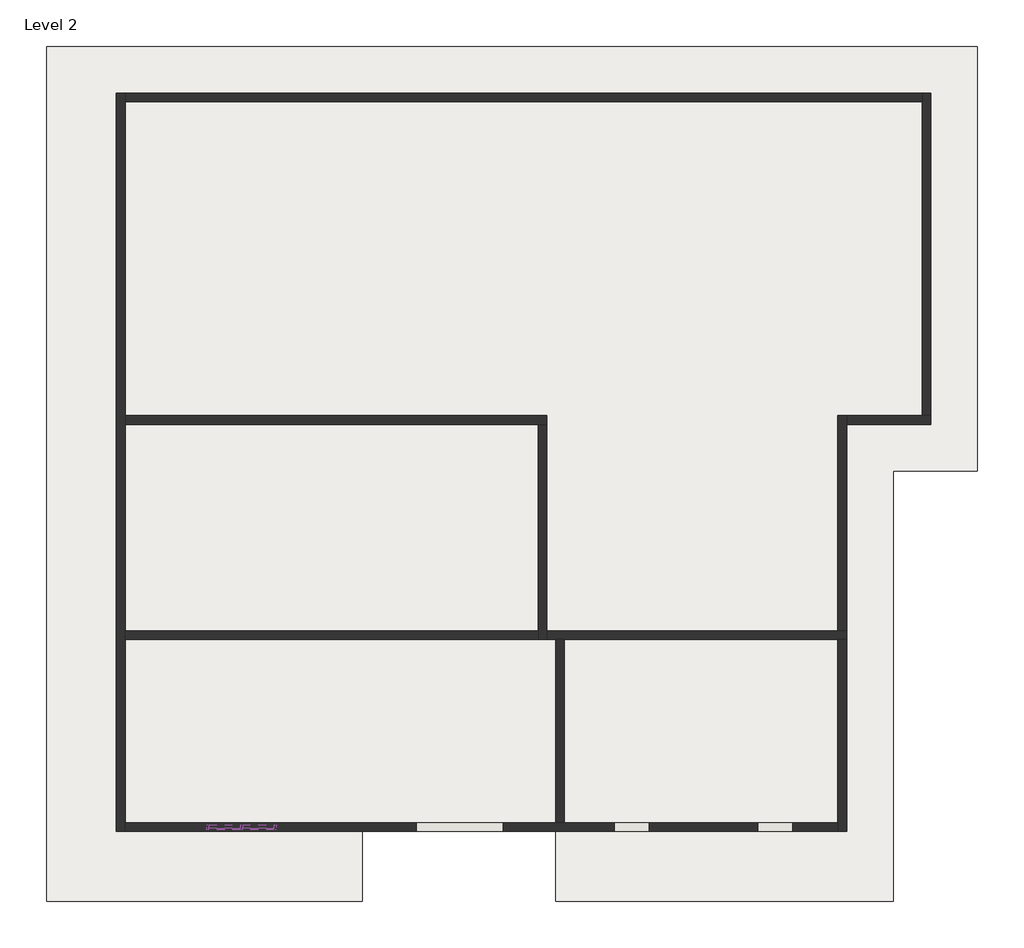
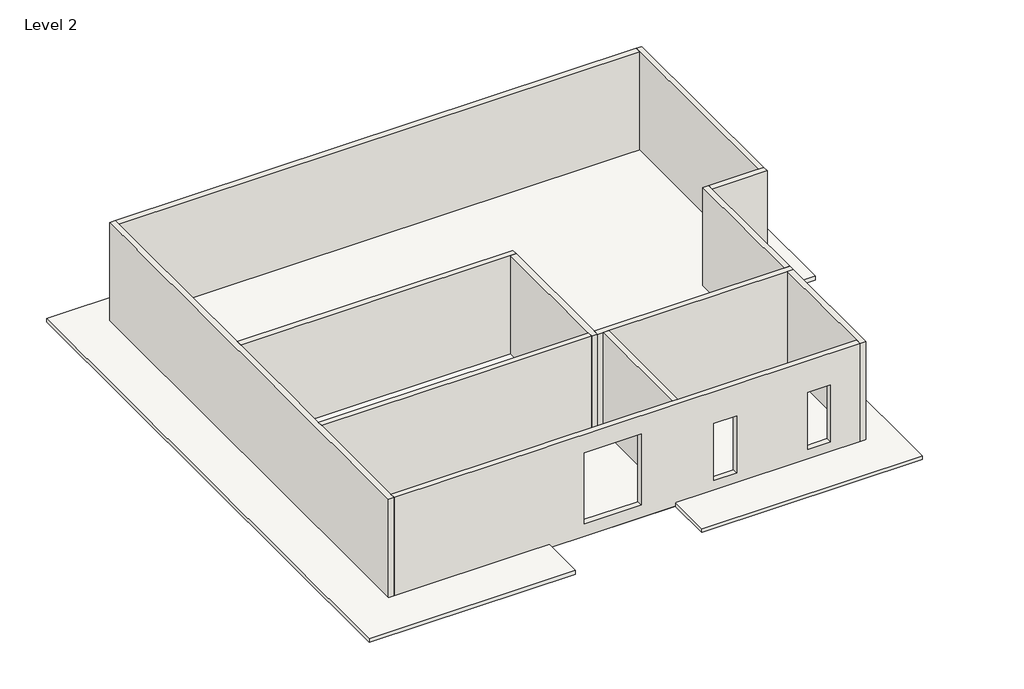
# One storey: 12 walls, 7 members, 4 plates, 1 roof.
"""IFC4 building model written with IfcOpenShell, lengths in millimetres."""

from ifc_helpers import new_model, si_unit, frame, origin, place, context, project, spatial, polyline, outline, extrude, faceted_brep, transform, mapped, element, save
from components import member_c17f1be2, member_2db96224, member_1ab8d6f1, system_panel_glazed_bec4471e, system_panel_glazed_61df8711, system_panel_glazed_48f0744a

model = new_model("IFC4")

# Units and contexts
model_context = context("Model", 3, world=origin())
ifc_project = project(units=[si_unit("LENGTHUNIT", "METRE", prefix="MILLI")], contexts=[model_context])

# Site, building, storey
site = spatial("IfcSite", under=ifc_project)
building = spatial("IfcBuilding", under=site)
storey = spatial("IfcBuildingStorey", under=building, Name="Level 2", Elevation=4165.6)

# Members
placement = place(None, origin())
member_shape = member_c17f1be2(model_context)
element("IfcMember", 1, ObjectType="Rectangular Mullion : 2.5\" x 5\" rectangular", at=placement, inside=storey, context=model_context, shape_type="MappedRepresentation", body=[
    mapped(member_shape, transform((-11225.4059085, -2978.2585517, 7874.0), x_axis=(0.0, 0.0, 1.0), y_axis=(0.0, 1.0, 0.0), z_axis=(-1.0, 0.0, 0.0))),
])
element("IfcMember", 2, ObjectType="Rectangular Mullion : 2.5\" x 5\" rectangular", at=placement, inside=storey, context=model_context, shape_type="MappedRepresentation", body=[
    mapped(member_shape, transform((-10342.7559085, -2978.2585517, 7874.0), x_axis=(0.0, 0.0, 1.0), y_axis=(0.0, 1.0, 0.0), z_axis=(-1.0, 0.0, 0.0))),
])
element("IfcMember", 3, ObjectType="Rectangular Mullion : 2.5\" x 5\" rectangular", at=placement, inside=storey, context=model_context, shape_type="MappedRepresentation", body=[
    mapped(member_shape, transform((-9523.6059085, -2978.2585517, 5689.6), x_axis=(0.0, 0.0, -1.0), y_axis=(0.0, 1.0, 0.0), z_axis=(1.0, 0.0, 0.0))),
])
element("IfcMember", 4, ObjectType="Rectangular Mullion : 2.5\" x 5\" rectangular", at=placement, inside=storey, context=model_context, shape_type="MappedRepresentation", body=[
    mapped(member_shape, transform((-10406.2559085, -2978.2585517, 5689.6), x_axis=(0.0, 0.0, -1.0), y_axis=(0.0, 1.0, 0.0), z_axis=(1.0, 0.0, 0.0))),
])
member_2_shape = member_2db96224(model_context)
element("IfcMember", 5, ObjectType="Rectangular Mullion : 2.5\" x 5\" rectangular", at=placement, inside=storey, context=model_context, shape_type="MappedRepresentation", body=[
    mapped(member_2_shape, transform((-10374.5059085, -2978.2585517, 5689.6), x_axis=(-1.0, 0.0, 0.0), y_axis=(0.0, 1.0, 0.0), z_axis=(0.0, 0.0, -1.0))),
])
member_3_shape = member_1ab8d6f1(model_context)
element("IfcMember", 6, ObjectType="Rectangular Mullion : 2.5\" x 5\" rectangular", at=placement, inside=storey, context=model_context, shape_type="MappedRepresentation", body=[
    mapped(member_3_shape, transform((-9460.1059085, -2978.2585517, 7874.0), x_axis=(1.0, 0.0, 0.0), y_axis=(0.0, 1.0, 0.0), z_axis=(0.0, 0.0, 1.0))),
])
element("IfcMember", 7, ObjectType="Rectangular Mullion : 2.5\" x 5\" rectangular", at=placement, inside=storey, context=model_context, shape_type="MappedRepresentation", body=[
    mapped(member_3_shape, transform((-11288.9059085, -2978.2585517, 5689.6), x_axis=(-1.0, 0.0, 0.0), y_axis=(0.0, 1.0, 0.0), z_axis=(0.0, 0.0, -1.0))),
])

# Plates
system_panel_glazed_shape = system_panel_glazed_bec4471e(model_context)
element("IfcPlate", 8, ObjectType="System Panel : Glazed", at=placement, inside=storey, context=model_context, shape_type="MappedRepresentation", body=[
    mapped(system_panel_glazed_shape, transform((-9933.1809085, -2978.2585517, 5753.1), x_axis=(-1.0, 0.0, 0.0), y_axis=(0.0, -1.0, 0.0), z_axis=(0.0, 0.0, 1.0))),
])
element("IfcPlate", 9, ObjectType="System Panel : Glazed", at=placement, inside=storey, context=model_context, shape_type="MappedRepresentation", body=[
    mapped(system_panel_glazed_shape, transform((-10815.8309085, -2978.2585517, 5753.1), x_axis=(-1.0, 0.0, 0.0), y_axis=(0.0, -1.0, 0.0), z_axis=(0.0, 0.0, 1.0))),
])
system_panel_glazed_2_shape = system_panel_glazed_61df8711(model_context)
element("IfcPlate", 10, ObjectType="System Panel : Glazed", at=placement, inside=storey, context=model_context, shape_type="MappedRepresentation", body=[
    mapped(system_panel_glazed_2_shape, transform((-4583.3059085, -2978.2585517, 4165.6), x_axis=(1.0, 0.0, 0.0), y_axis=(0.0, 1.0, 0.0), z_axis=(0.0, 0.0, 1.0))),
])
system_panel_glazed_3_shape = system_panel_glazed_48f0744a(model_context)
element("IfcPlate", 11, ObjectType="System Panel : Glazed", at=placement, inside=storey, context=model_context, shape_type="MappedRepresentation", body=[
    mapped(system_panel_glazed_3_shape, transform((-4583.3059085, -2978.2585517, 4165.6), x_axis=(1.0, 0.0, 0.0), y_axis=(0.0, 1.0, 0.0), z_axis=(0.0, 0.0, 1.0))),
])

# Roof
element("IfcRoof", 12, ObjectType="6\"", at=placement, inside=storey, context=model_context, shape_type="SweptSolid", body=[
    extrude(outline(polyline([(-15479.9059085, 17481.4414483), (8904.0940915, 17481.4414483), (8904.0940915, 6356.2414483), (6694.2940915, 6356.2414483), (6694.2940915, -4921.3585517), (-2144.9059085, -4921.3585517), (-2144.9059085, -3092.5585517), (-7212.2059085, -3092.5585517), (-7212.2059085, -4921.3585517), (-15479.9059085, -4921.3585517), (-15479.9059085, 17481.4414483)])), frame((0.0, 0.0, 4165.6), z_axis=(0.0, 0.0, 1.0), x_axis=(1.0, 0.0, 0.0)), (0.0, 0.0, 1.0), 152.4),
])

# Walls
element("IfcWall", 13, ObjectType="9\" wall", at=placement, inside=storey, context=model_context, shape_type="Brep", body=[
    faceted_brep([(-13651.1059085, 16262.2414483, 4165.6), (-13651.1059085, -3092.5585517, 4165.6), (-13651.1059085, -3092.5585517, 8483.6), (-13651.1059085, 4832.2414483, 8483.6), (-13651.1059085, 4946.5414483, 8483.6), (-13651.1059085, 14319.1414483, 8483.6), (-13651.1059085, 14433.4414483, 8483.6), (-13651.1059085, 16262.2414483, 8483.6), (-13422.5059085, 16262.2414483, 4165.6), (-13422.5059085, 16262.2414483, 8483.6), (-13422.5059085, 16033.6414483, 8483.6), (-13422.5059085, 14433.4414483, 8483.6), (-13422.5059085, 14319.1414483, 8483.6), (-13422.5059085, 7804.0414483, 8483.6), (-13422.5059085, 7575.4414483, 8483.6), (-13422.5059085, 4946.5414483, 8483.6), (-13422.5059085, 4832.2414483, 8483.6), (-13422.5059085, 2165.2414483, 8483.6), (-13422.5059085, 1936.6414483, 8483.6), (-13422.5059085, -2863.9585517, 8483.6), (-13422.5059085, -3092.5585517, 8483.6), (-13422.5059085, -3092.5585517, 4165.6), (-13422.5059085, -2863.9585517, 4165.6), (-13422.5059085, 1936.6414483, 4165.6), (-13422.5059085, 2165.2414483, 4165.6), (-13422.5059085, 7575.4414483, 4165.6), (-13422.5059085, 7804.0414483, 4165.6), (-13422.5059085, 16033.6414483, 4165.6)], [[[0, 1, 2, 3, 4, 5, 6, 7]], [[8, 9, 10, 11, 12, 13, 14, 15, 16, 17, 18, 19, 20, 21, 22, 23, 24, 25, 26, 27]], [[1, 0, 8, 27, 26, 25, 24, 23, 22, 21]], [[7, 6, 5, 4, 3, 2, 20, 19, 18, 17, 16, 15, 14, 13, 12, 11, 10, 9]], [[2, 1, 21, 20]], [[0, 7, 9, 8]]]),
])
element("IfcWall", 14, ObjectType="9\" wall", at=placement, inside=storey, context=model_context, shape_type="Brep", body=[
    faceted_brep([(-13422.5059085, 7575.4414483, 4165.6), (-2602.1059085, 7575.4414483, 4165.6), (-2373.5059085, 7575.4414483, 4165.6), (-2373.5059085, 7575.4414483, 8483.6), (-2602.1059085, 7575.4414483, 8483.6), (-13422.5059085, 7575.4414483, 8483.6), (-13422.5059085, 7804.0414483, 4165.6), (-13422.5059085, 7804.0414483, 8483.6), (-2373.5059085, 7804.0414483, 8483.6), (-2373.5059085, 7804.0414483, 4165.6)], [[[0, 1, 2, 3, 4, 5]], [[6, 7, 8, 9]], [[2, 1, 0, 6, 9]], [[5, 4, 3, 8, 7]], [[0, 5, 7, 6]], [[3, 2, 9, 8]]]),
])
element("IfcWall", 15, ObjectType="9\" wall", at=placement, inside=storey, context=model_context, shape_type="Brep", body=[
    faceted_brep([(-2602.1059085, 7575.4414483, 4165.6), (-2602.1059085, 2165.2414483, 4165.6), (-2602.1059085, 1936.6414483, 4165.6), (-2602.1059085, 1936.6414483, 8483.6), (-2602.1059085, 2165.2414483, 8483.6), (-2602.1059085, 7575.4414483, 8483.6), (-2373.5059085, 7575.4414483, 4165.6), (-2373.5059085, 7575.4414483, 8483.6), (-2373.5059085, 2165.2414483, 8483.6), (-2373.5059085, 1936.6414483, 8483.6), (-2373.5059085, 1936.6414483, 4165.6), (-2373.5059085, 2165.2414483, 4165.6)], [[[0, 1, 2, 3, 4, 5]], [[6, 7, 8, 9, 10, 11]], [[2, 1, 0, 6, 11, 10]], [[5, 4, 3, 9, 8, 7]], [[0, 5, 7, 6]], [[3, 2, 10, 9]]]),
])
element("IfcWall", 16, ObjectType="9\" wall", at=placement, inside=storey, context=model_context, shape_type="Brep", body=[
    faceted_brep([(-2373.5059085, 1936.6414483, 4165.6), (-2144.9059085, 1936.6414483, 4165.6), (-1916.3059085, 1936.6414483, 4165.6), (5246.4940915, 1936.6414483, 4165.6), (5475.0940915, 1936.6414483, 4165.6), (5475.0940915, 1936.6414483, 8483.6), (5246.4940915, 1936.6414483, 8483.6), (-1916.3059085, 1936.6414483, 8483.6), (-2144.9059085, 1936.6414483, 8483.6), (-2373.5059085, 1936.6414483, 8483.6), (-2373.5059085, 2165.2414483, 4165.6), (-2373.5059085, 2165.2414483, 8483.6), (5246.4940915, 2165.2414483, 8483.6), (5475.0940915, 2165.2414483, 8483.6), (5475.0940915, 2165.2414483, 4165.6), (5246.4940915, 2165.2414483, 4165.6)], [[[0, 1, 2, 3, 4, 5, 6, 7, 8, 9]], [[10, 11, 12, 13, 14, 15]], [[4, 3, 2, 1, 0, 10, 15, 14]], [[9, 8, 7, 6, 5, 13, 12, 11]], [[0, 9, 11, 10]], [[5, 4, 14, 13]]]),
])
element("IfcWall", 17, ObjectType="9\" wall", at=placement, inside=storey, context=model_context, shape_type="Brep", body=[
    faceted_brep([(5475.0940915, 2165.2414483, 4165.6), (5475.0940915, 7575.4414483, 4165.6), (5475.0940915, 7804.0414483, 4165.6), (5475.0940915, 7804.0414483, 8483.6), (5475.0940915, 7575.4414483, 8483.6), (5475.0940915, 2165.2414483, 8483.6), (5246.4940915, 2165.2414483, 4165.6), (5246.4940915, 2165.2414483, 8483.6), (5246.4940915, 7804.0414483, 8483.6), (5246.4940915, 7804.0414483, 4165.6)], [[[0, 1, 2, 3, 4, 5]], [[6, 7, 8, 9]], [[2, 1, 0, 6, 9]], [[5, 4, 3, 8, 7]], [[0, 5, 7, 6]], [[3, 2, 9, 8]]]),
])
element("IfcWall", 18, ObjectType="9\" wall", at=placement, inside=storey, context=model_context, shape_type="Brep", body=[
    faceted_brep([(-2602.1059085, 2165.2414483, 4165.6), (-13422.5059085, 2165.2414483, 4165.6), (-13422.5059085, 2165.2414483, 8483.6), (-7339.2059085, 2165.2414483, 8483.6), (-7237.6059085, 2165.2414483, 8483.6), (-2602.1059085, 2165.2414483, 8483.6), (-2602.1059085, 1936.6414483, 4165.6), (-2602.1059085, 1936.6414483, 8483.6), (-7237.6059085, 1936.6414483, 8483.6), (-7339.2059085, 1936.6414483, 8483.6), (-13422.5059085, 1936.6414483, 8483.6), (-13422.5059085, 1936.6414483, 4165.6)], [[[0, 1, 2, 3, 4, 5]], [[6, 7, 8, 9, 10, 11]], [[1, 0, 6, 11]], [[5, 4, 3, 2, 10, 9, 8, 7]], [[0, 5, 7, 6]], [[2, 1, 11, 10]]]),
])
element("IfcWall", 19, ObjectType="9\" wall", at=placement, inside=storey, context=model_context, shape_type="Brep", body=[
    faceted_brep([(5246.4940915, 1936.6414483, 4165.6), (5246.4940915, -2863.9585517, 4165.6), (5246.4940915, -3092.5585517, 4165.6), (5246.4940915, -3092.5585517, 8483.6), (5246.4940915, -2863.9585517, 8483.6), (5246.4940915, 1936.6414483, 8483.6), (5475.0940915, 1936.6414483, 4165.6), (5475.0940915, 1936.6414483, 8483.6), (5475.0940915, -3092.5585517, 8483.6), (5475.0940915, -3092.5585517, 4165.6)], [[[0, 1, 2, 3, 4, 5]], [[6, 7, 8, 9]], [[2, 1, 0, 6, 9]], [[5, 4, 3, 8, 7]], [[0, 5, 7, 6]], [[3, 2, 9, 8]]]),
])
element("IfcWall", 20, ObjectType="9\" wall", at=placement, inside=storey, context=model_context, shape_type="Brep", body=[
    faceted_brep([(5246.4940915, -2863.9585517, 4165.6), (-1916.3059085, -2863.9585517, 4165.6), (-2144.9059085, -2863.9585517, 4165.6), (-13422.5059085, -2863.9585517, 4165.6), (-13422.5059085, -2863.9585517, 8483.6), (-7339.2059085, -2863.9585517, 8483.6), (-7237.6059085, -2863.9585517, 8483.6), (-2144.9059085, -2863.9585517, 8483.6), (-1916.3059085, -2863.9585517, 8483.6), (5246.4940915, -2863.9585517, 8483.6), (-5802.5059085, -2863.9585517, 7710.9437287), (-5802.5059085, -2863.9585517, 4699.5804549), (-3516.5059085, -2863.9585517, 4699.5804549), (-3516.5059085, -2863.9585517, 7710.9437287), (-608.2059085, -2863.9585517, 7128.8390806), (-608.2059085, -2863.9585517, 4716.8478077), (306.1940915, -2863.9585517, 4716.8478077), (306.1940915, -2863.9585517, 7128.8390806), (4065.3940915, -2863.9585517, 4716.8478077), (4065.3940915, -2863.9585517, 7128.8390806), (3150.9940915, -2863.9585517, 7128.8390806), (3150.9940915, -2863.9585517, 4716.8478077), (-13422.5059085, -3092.5585517, 4165.6), (5246.4940915, -3092.5585517, 4165.6), (5246.4940915, -3092.5585517, 8483.6), (-7237.6059085, -3092.5585517, 8483.6), (-7339.2059085, -3092.5585517, 8483.6), (-13422.5059085, -3092.5585517, 8483.6), (-5802.5059085, -3092.5585517, 4699.5804549), (-5802.5059085, -3092.5585517, 7710.9437287), (-3516.5059085, -3092.5585517, 7710.9437287), (-3516.5059085, -3092.5585517, 4699.5804549), (-608.2059085, -3092.5585517, 4716.8478077), (-608.2059085, -3092.5585517, 7128.8390806), (306.1940915, -3092.5585517, 7128.8390806), (306.1940915, -3092.5585517, 4716.8478077), (4065.3940915, -3092.5585517, 7128.8390806), (4065.3940915, -3092.5585517, 4716.8478077), (3150.9940915, -3092.5585517, 4716.8478077), (3150.9940915, -3092.5585517, 7128.8390806)], [[[0, 1, 2, 3, 4, 5, 6, 7, 8, 9], [10, 11, 12, 13], [14, 15, 16, 17], [18, 19, 20, 21]], [[22, 23, 24, 25, 26, 27], [28, 29, 30, 31], [32, 33, 34, 35], [36, 37, 38, 39]], [[3, 2, 1, 0, 23, 22]], [[9, 8, 7, 6, 5, 4, 27, 26, 25, 24]], [[0, 9, 24, 23]], [[4, 3, 22, 27]], [[28, 11, 10, 29]], [[29, 10, 13, 30]], [[30, 13, 12, 31]], [[11, 28, 31, 12]], [[32, 15, 14, 33]], [[33, 14, 17, 34]], [[34, 17, 16, 35]], [[15, 32, 35, 16]], [[18, 37, 36, 19]], [[19, 36, 39, 20]], [[20, 39, 38, 21]], [[37, 18, 21, 38]]]),
])
element("IfcWall", 21, ObjectType="9\" wall", at=placement, inside=storey, context=model_context, shape_type="SweptSolid", body=[
    extrude(outline(polyline([(-1916.3059085, 1936.6414483), (-1916.3059085, -2863.9585517), (-2144.9059085, -2863.9585517), (-2144.9059085, 1936.6414483), (-1916.3059085, 1936.6414483)])), frame((0.0, 0.0, 4165.6), z_axis=(0.0, 0.0, 1.0), x_axis=(1.0, 0.0, 0.0)), (0.0, 0.0, 1.0), 4318.0),
])
element("IfcWall", 22, ObjectType="9\" wall", at=placement, inside=storey, context=model_context, shape_type="Brep", body=[
    faceted_brep([(5475.0940915, 7575.4414483, 4165.6), (7684.8940915, 7575.4414483, 4165.6), (7684.8940915, 7575.4414483, 8483.6), (5475.0940915, 7575.4414483, 8483.6), (5475.0940915, 7804.0414483, 4165.6), (5475.0940915, 7804.0414483, 8483.6), (7456.2940915, 7804.0414483, 8483.6), (7684.8940915, 7804.0414483, 8483.6), (7684.8940915, 7804.0414483, 4165.6), (7456.2940915, 7804.0414483, 4165.6)], [[[0, 1, 2, 3]], [[4, 5, 6, 7, 8, 9]], [[1, 0, 4, 9, 8]], [[3, 2, 7, 6, 5]], [[0, 3, 5, 4]], [[2, 1, 8, 7]]]),
])
element("IfcWall", 23, ObjectType="9\" wall", at=placement, inside=storey, context=model_context, shape_type="Brep", body=[
    faceted_brep([(7684.8940915, 7804.0414483, 4165.6), (7684.8940915, 16262.2414483, 4165.6), (7684.8940915, 16262.2414483, 8483.6), (7684.8940915, 7804.0414483, 8483.6), (7456.2940915, 7804.0414483, 4165.6), (7456.2940915, 7804.0414483, 8483.6), (7456.2940915, 16033.6414483, 8483.6), (7456.2940915, 16262.2414483, 8483.6), (7456.2940915, 16262.2414483, 4165.6), (7456.2940915, 16033.6414483, 4165.6)], [[[0, 1, 2, 3]], [[4, 5, 6, 7, 8, 9]], [[1, 0, 4, 9, 8]], [[3, 2, 7, 6, 5]], [[0, 3, 5, 4]], [[2, 1, 8, 7]]]),
])
element("IfcWall", 24, ObjectType="9\" wall", at=placement, inside=storey, context=model_context, shape_type="SweptSolid", body=[
    extrude(outline(polyline([(-13422.5059085, 16262.2414483), (7456.2940915, 16262.2414483), (7456.2940915, 16033.6414483), (-13422.5059085, 16033.6414483), (-13422.5059085, 16262.2414483)])), frame((0.0, 0.0, 4165.6), z_axis=(0.0, 0.0, 1.0), x_axis=(1.0, 0.0, 0.0)), (0.0, 0.0, 1.0), 4318.0),
])

save(model, "model.ifc")

# Revit data of these elements
# Type "Rectangular Mullion : 2.5\" x 5\" rectangular"
#   built-in parameter 1007304 = 0.416667 (stored number, unit not read)
#   built-in parameter 1007301 = 0.104167 (stored number, unit not read)
#   built-in parameter 1007300 = 0.104167 (stored number, unit not read)
# Type "System Panel : Glazed"
#   Construction Type Id = "GSP4R"
#   Analytic Construction = "1/8 in Pilkington single glazing"
#   Visual Light Transmittance = 0.9
#   Solar Heat Gain Coefficient = 0.86
#   Heat Transfer Coefficient (U) = 1.18115 BTU/(h·ft²·°F)
#   Define Thermal Properties by = 1
# Type "6\""
#   Assembly Code = "B1020"
#   Layers, outside or top first: 0' - 6" "warm colour" (function 1)
# Type "9\" wall"
#   Assembly Code = "B2010"
#   Layers, outside or top first: 0' - 9" "warm colour" (function 1)
# Elements 1, 2, 3, 4, 5, 6, 7 (IfcMember, "Rectangular Mullion : 2.5\" x 5\" rectangular")
#   Phase Created = New Construction
# Elements 8, 9, 10, 11 (IfcPlate, "System Panel : Glazed")
#   Phase Created = New Construction
#   Materials on its faces: "Glass"
# Element 12 (IfcRoof, "6\"")
#   built-in parameter 1001705 = 14.1667 (stored number, unit not read)
#   built-in parameter 1001701 = 0 (stored number, unit not read)
#   built-in parameter 1001710 = 33615
#   Phase Created = New Construction
#   Materials on its faces: "warm colour"
# Elements 13, 14, 15, 16, 17, 18, 19, 20, 21, 22, 23, 24 (IfcWall, "9\" wall")
#   Top Offset = 1' - 0"
#   Base Offset = 0' - 0"
#   Unconnected Height = 14' - 2"
#   wall height = 14' - 2"
#   Phase Created = New Construction
#   Base Constraint = Level 2
#   Materials on its faces: "warm colour"
# Materials
#   "warm colour": class "Generic", colour RGB 120 120 120, transparency 0, Cost = 0
#   "Glass": class "Glass", colour RGB 0 128 192, transparency 0.75, Description = "Soda Lime Glass", Cost = 0
